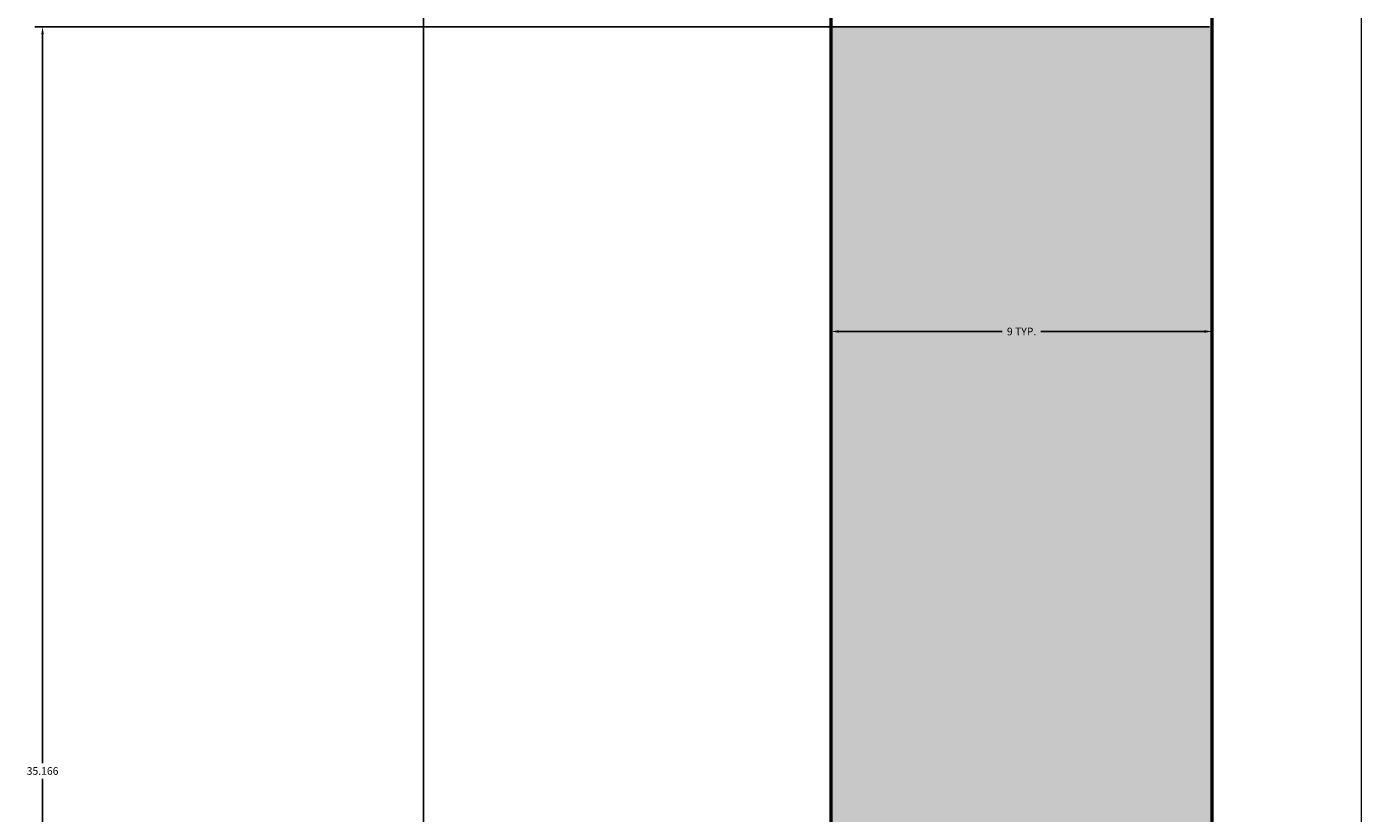
# Model space of a CAD drawing. Units: inches. Extents: x 2231 to 2461, y 2045 to 2455.
# Tile 37 of 95: x 2231 to 2262, y 2203 to 2222. Entities that reach past the tile are written whole.
import ezdxf

# ---------------------------------------------------------------- set-up
doc = ezdxf.new("R2010")
doc.units = ezdxf.units.IN
for name, color, linetype, lineweight in [('A-ANNO-DIMS', 2, 'Continuous', 18), ('A-FURN', 9, 'Continuous', 18), ('A-WALL', 7, 'Continuous', 50)]:
    doc.layers.add(name, color=color, linetype=linetype, lineweight=lineweight)
doc.layers.add('A-WALL-PATT', color=18, linetype='Continuous', lineweight=13, true_color=0x000000)
doc.styles.get("Standard").update_dxf_attribs({"font": 'arial.ttf'})
doc.dimstyles.get("Standard").update_dxf_attribs({"dimtxt": 0.18, "dimasz": 0.18, "dimexe": 0.18, "dimexo": 0.0625, "dimgap": 0.09, "dimtad": 0, "dimtih": 1, "dimtoh": 1, "dimdec": 4, "dimzin": 0, "dimdsep": 46, "dimtxsty": 'Standard', "dimcen": 0.09, "dimadec": 0, "dimazin": 0, "dimtfac": 1, "dimtdec": 4, "dimtofl": 0, "dimtmove": 0, "dimatfit": 3, "dimfxl": 1, "dimtolj": 1, "dimtzin": 0, "dimarcsym": 0})

# ---------------------------------------------------------------- blocks, each defined once
blk = doc.blocks.new('*D16')
at = {"layer": 'A-ANNO-DIMS', "color": 0, "lineweight": -2, "transparency": 16777216}
for p, q in [((2249.794, 2221.937), (2249.794, 2214.619)), ((2258.794, 2221.937), (2258.794, 2214.619)), ((2249.974, 2214.799), (2253.835, 2214.799)), ((2258.614, 2214.799), (2254.752, 2214.799))]:
    blk.add_line(p, q, dxfattribs=at)
at = {"layer": 'A-ANNO-DIMS', "color": 0, "transparency": 16777216}
for points in [[(2249.974, 2214.829), (2249.974, 2214.769), (2249.794, 2214.799)], [(2258.614, 2214.829), (2258.614, 2214.769), (2258.794, 2214.799)]]:
    blk.add_solid(points, dxfattribs=at)
at = {"layer": 'Defpoints', "color": 0, "transparency": 16777216}
for p in [(2249.794, 2221.999), (2258.794, 2221.999), (2258.794, 2214.799)]:
    blk.add_point(p, dxfattribs=at)
at = {"layer": 'A-ANNO-DIMS', "color": 0, "transparency": 16777216, "insert": (2254.294, 2214.799), "char_height": 0.18, "attachment_point": 5}
blk.add_mtext('\\A1;9 TYP.', dxfattribs=at)
blk = doc.blocks.new('*D39')
at = {"layer": 'A-ANNO-DIMS', "color": 0, "lineweight": -2, "transparency": 16777216}
for p, q in [((2258.731, 2221.999), (2230.981, 2221.999)), ((2231.161, 2221.819), (2231.161, 2204.598)), ((2231.161, 2187.013), (2231.161, 2204.234)), ((2258.731, 2186.833), (2230.981, 2186.833))]:
    blk.add_line(p, q, dxfattribs=at)
at = {"layer": 'A-ANNO-DIMS', "color": 0, "transparency": 16777216}
for points in [[(2231.131, 2221.819), (2231.191, 2221.819), (2231.161, 2221.999)], [(2231.131, 2187.013), (2231.191, 2187.013), (2231.161, 2186.833)]]:
    blk.add_solid(points, dxfattribs=at)
at = {"layer": 'Defpoints', "color": 0, "transparency": 16777216}
for p in [(2231.161, 2221.999), (2258.794, 2221.999), (2258.794, 2186.833)]:
    blk.add_point(p, dxfattribs=at)
at = {"layer": 'A-ANNO-DIMS', "color": 0, "transparency": 16777216, "insert": (2231.161, 2204.416), "char_height": 0.18, "attachment_point": 5}
blk.add_mtext('\\A1;35.166', dxfattribs=at)
blk = doc.blocks.new('*D40')
at = {"layer": 'A-ANNO-DIMS', "color": 0, "lineweight": -2, "transparency": 16777216}
for p, q in [((2258.731, 2302.833), (2239.981, 2302.833)), ((2240.161, 2302.653), (2240.161, 2245.015)), ((2240.161, 2187.013), (2240.161, 2244.651)), ((2258.731, 2186.833), (2239.981, 2186.833))]:
    blk.add_line(p, q, dxfattribs=at)
at = {"layer": 'A-ANNO-DIMS', "color": 0, "transparency": 16777216}
for points in [[(2240.131, 2302.653), (2240.191, 2302.653), (2240.161, 2302.833)], [(2240.131, 2187.013), (2240.191, 2187.013), (2240.161, 2186.833)]]:
    blk.add_solid(points, dxfattribs=at)
at = {"layer": 'Defpoints', "color": 0, "transparency": 16777216}
for p in [(2240.161, 2302.833), (2258.794, 2302.833), (2258.794, 2186.833)]:
    blk.add_point(p, dxfattribs=at)
at = {"layer": 'A-ANNO-DIMS', "color": 0, "transparency": 16777216, "insert": (2240.161, 2244.833), "char_height": 0.18, "attachment_point": 5}
blk.add_mtext('\\A1;116', dxfattribs=at)
blk = doc.blocks.new('*D47')
at = {"layer": 'A-ANNO-DIMS', "color": 0, "lineweight": -2, "transparency": 16777216}
for p, q in [((2258.794, 2182.895), (2258.794, 2454.645)), ((2258.974, 2454.465), (2276.575, 2454.465)), ((2294.614, 2454.465), (2277.012, 2454.465)), ((2294.794, 2182.895), (2294.794, 2454.645))]:
    blk.add_line(p, q, dxfattribs=at)
at = {"layer": 'A-ANNO-DIMS', "color": 0, "transparency": 16777216}
for points in [[(2258.974, 2454.495), (2258.974, 2454.435), (2258.794, 2454.465)], [(2294.614, 2454.495), (2294.614, 2454.435), (2294.794, 2454.465)]]:
    blk.add_solid(points, dxfattribs=at)
at = {"layer": 'Defpoints', "color": 0, "transparency": 16777216}
for p in [(2294.794, 2454.465), (2258.794, 2182.833), (2294.794, 2182.833)]:
    blk.add_point(p, dxfattribs=at)
at = {"layer": 'A-ANNO-DIMS', "color": 0, "transparency": 16777216, "insert": (2276.794, 2454.465), "char_height": 0.18, "attachment_point": 5}
blk.add_mtext('\\A1;36', dxfattribs=at)
blk = doc.blocks.new('*D51')
at = {"layer": 'A-ANNO-DIMS', "color": 0, "lineweight": -2, "transparency": 16777216}
for p, q in [((2258.794, 2306.77), (2258.794, 2044.803)), ((2330.794, 2306.77), (2330.794, 2044.803)), ((2258.974, 2044.983), (2294.576, 2044.983)), ((2330.614, 2044.983), (2295.011, 2044.983))]:
    blk.add_line(p, q, dxfattribs=at)
at = {"layer": 'A-ANNO-DIMS', "color": 0, "transparency": 16777216}
for points in [[(2258.974, 2045.013), (2258.974, 2044.953), (2258.794, 2044.983)], [(2330.614, 2045.013), (2330.614, 2044.953), (2330.794, 2044.983)]]:
    blk.add_solid(points, dxfattribs=at)
at = {"layer": 'Defpoints', "color": 0, "transparency": 16777216}
for p in [(2258.794, 2306.833), (2330.794, 2306.833), (2330.794, 2044.983)]:
    blk.add_point(p, dxfattribs=at)
at = {"layer": 'A-ANNO-DIMS', "color": 0, "transparency": 16777216, "insert": (2294.794, 2044.983), "char_height": 0.18, "attachment_point": 5}
blk.add_mtext('\\A1;72', dxfattribs=at)

msp = doc.modelspace()

# ---------------------------------------------------------------- hatches: boundary and pattern name
at = {"layer": 'A-WALL-PATT'}
h = msp.add_hatch(color=256, dxfattribs=at)
h.dxf.hatch_style = 1
h.paths.add_polyline_path([(2441.7935, 2269.1535), (2432.7935, 2269.1535), (2432.7935, 2186.8328), (2396.7935, 2186.8328), (2396.7935, 2286.8328), (2394.7935, 2286.8328), (2394.7935, 2186.8328), (2334.7935, 2186.8328), (2334.7935, 2182.8328), (2432.7935, 2182.8328), (2432.7935, 2072.8328), (2416.6639, 2072.8328), (2416.6639, 2063.8328), (2441.7935, 2063.8328)])
h.paths.add_polyline_path([(2368.6639, 2072.8328), (2367.04, 2072.8328), (2330.7942, 2072.8328), (2330.7397, 2063.8328), (2368.6639, 2063.8328)])
h.paths.add_polyline_path([(2300.7392, 2068.3328), (2300.7392, 2072.8328), (2298.7935, 2072.8328), (2294.7935, 2072.8328), (2258.7935, 2072.8328), (2258.7935, 2120.8328), (2294.7935, 2120.8328), (2298.7935, 2120.8328), (2298.7935, 2128.8328), (2294.7935, 2128.8328), (2294.7935, 2124.8328), (2258.7935, 2124.8328), (2258.7935, 2182.8328), (2294.7935, 2182.8328), (2294.7935, 2174.8328), (2298.7935, 2174.8328), (2298.7935, 2182.8328), (2304.7935, 2182.8328), (2304.7935, 2186.8328), (2258.7935, 2186.8328), (2258.7935, 2221.999), (2249.7935, 2221.999), (2249.7935, 2063.8328), (2300.7392, 2063.8328)])
h.paths.add_polyline_path([(2391.9338, 2435.8328), (2333.82, 2435.8328), (2333.82, 2426.8328), (2368.7935, 2426.8328), (2368.7935, 2374.9508), (2368.7935, 2370.8328), (2372.3935, 2370.8328), (2372.7935, 2370.8328), (2372.7935, 2426.8328), (2391.9338, 2426.8328)])
h.paths.add_polyline_path([(2441.7935, 2435.8328), (2415.9338, 2435.8328), (2415.9338, 2426.8328), (2432.7935, 2426.8328), (2432.7935, 2334.8328), (2372.7935, 2334.8328), (2372.7935, 2346.8328), (2368.7935, 2346.8328), (2368.7935, 2306.8328), (2360.7935, 2306.8328), (2360.7935, 2302.8328), (2368.7935, 2302.8328), (2372.7935, 2302.8328), (2372.7935, 2330.8328), (2432.7935, 2330.8328), (2432.7935, 2317.1535), (2441.7935, 2317.1535)])
h.paths.add_polyline_path([(2285.82, 2435.8328), (2249.7935, 2435.8328), (2249.7935, 2269.999), (2258.7935, 2269.999), (2258.7935, 2302.8328), (2318.8168, 2302.8328), (2330.7935, 2302.8328), (2330.7935, 2306.8328), (2258.7935, 2306.8328), (2258.7935, 2426.8328), (2285.82, 2426.8328)])

# ---------------------------------------------------------------- linework, layer by layer
at = {"layer": 'A-FURN'}
msp.add_line((2262.3207, 2255.1137), (2262.3207, 2195.1137), dxfattribs=at)
at = {"layer": 'A-WALL'}
msp.add_line((2258.7935, 2186.8328), (2258.7935, 2302.8328), dxfattribs=at)
msp.add_lwpolyline([(2300.7392, 2063.8328), (2249.7935, 2063.8328), (2249.7935, 2435.8328), (2441.7935, 2435.8328), (2441.7935, 2063.8328), (2330.7397, 2063.8328)], dxfattribs=at)

# ---------------------------------------------------------------- dimensions: what is measured, and where the dimension line sits
at = {"layer": 'A-ANNO-DIMS'}
for base, p1, p2, picture, middle in [((2294.7935, 2454.4653), (2258.7935, 2182.8328), (2294.7935, 2182.8328), '*D47', (2276.7935, 2454.4653)), ((2330.7935, 2044.9825), (2258.7935, 2306.8328), (2330.7935, 2306.8328), '*D51', (2294.7935, 2044.9825))]:
    dim = msp.add_linear_dim(base=base, p1=p1, p2=p2, dimstyle='Standard', override={"dimdec": 0, "dimlfac": 1, "dimrnd": 0, "dimzin": 0, "dimdsep": 46, "dimlunit": 2}, dxfattribs=at)
    dim.commit()
    dim.dimension.update_dxf_attribs({"geometry": picture, "text_midpoint": middle})
for base, p2, override, picture, middle in [((2240.161, 2302.8328), (2258.7935, 2302.8328), {"dimdec": 0, "dimlfac": 1, "dimrnd": 0, "dimzin": 0, "dimdsep": 46, "dimlunit": 2}, '*D40', (2240.161, 2244.8328)), ((2231.161, 2221.999), (2258.7935, 2221.999), {"dimdec": 3, "dimlfac": 1, "dimrnd": 0, "dimzin": 0, "dimdsep": 46, "dimlunit": 2}, '*D39', (2231.161, 2204.4159))]:
    dim = msp.add_linear_dim(base=base, p1=(2258.7935, 2186.8328), p2=p2, angle=90, dimstyle='Standard', override=override, dxfattribs=at)
    dim.commit()
    dim.dimension.update_dxf_attribs({"geometry": picture, "text_midpoint": middle})
dim = msp.add_linear_dim(base=(2258.7935, 2214.799), p1=(2249.7935, 2221.999), p2=(2258.7935, 2221.999), text='<> TYP.', dimstyle='Standard', override={"dimdec": 0, "dimlfac": 1, "dimrnd": 0, "dimzin": 0, "dimdsep": 46, "dimlunit": 2}, dxfattribs=at)
dim.commit()
dim.dimension.update_dxf_attribs({"geometry": '*D16', "text_midpoint": (2254.2935, 2214.799)})

doc.saveas('drawing.dxf')
